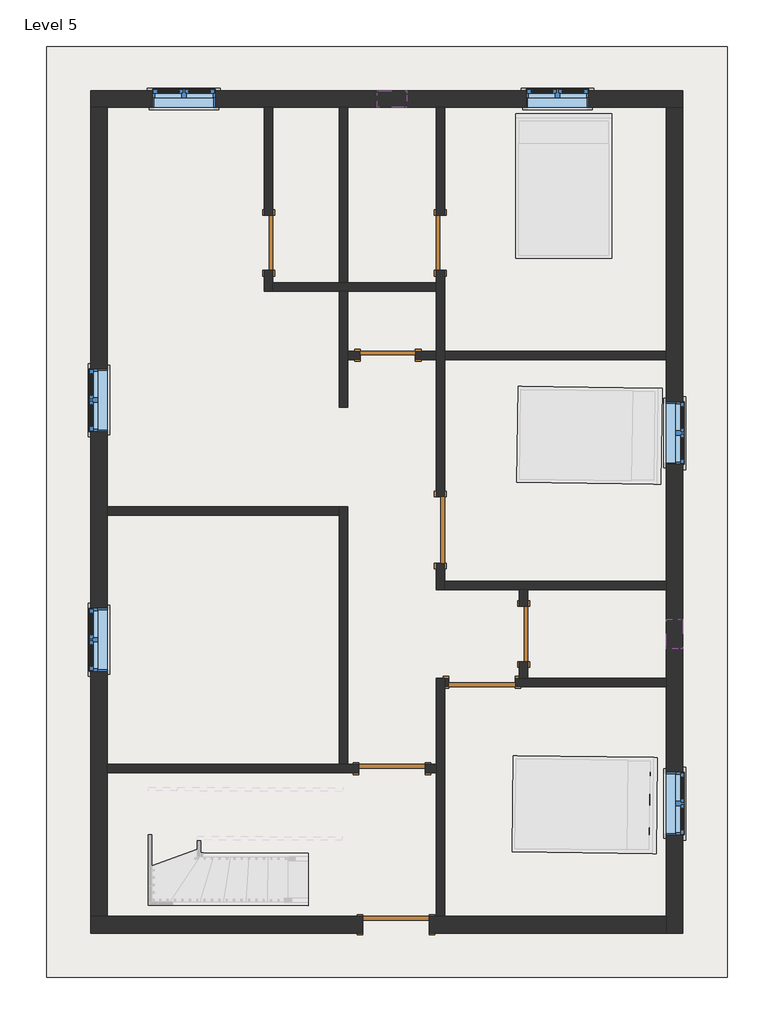
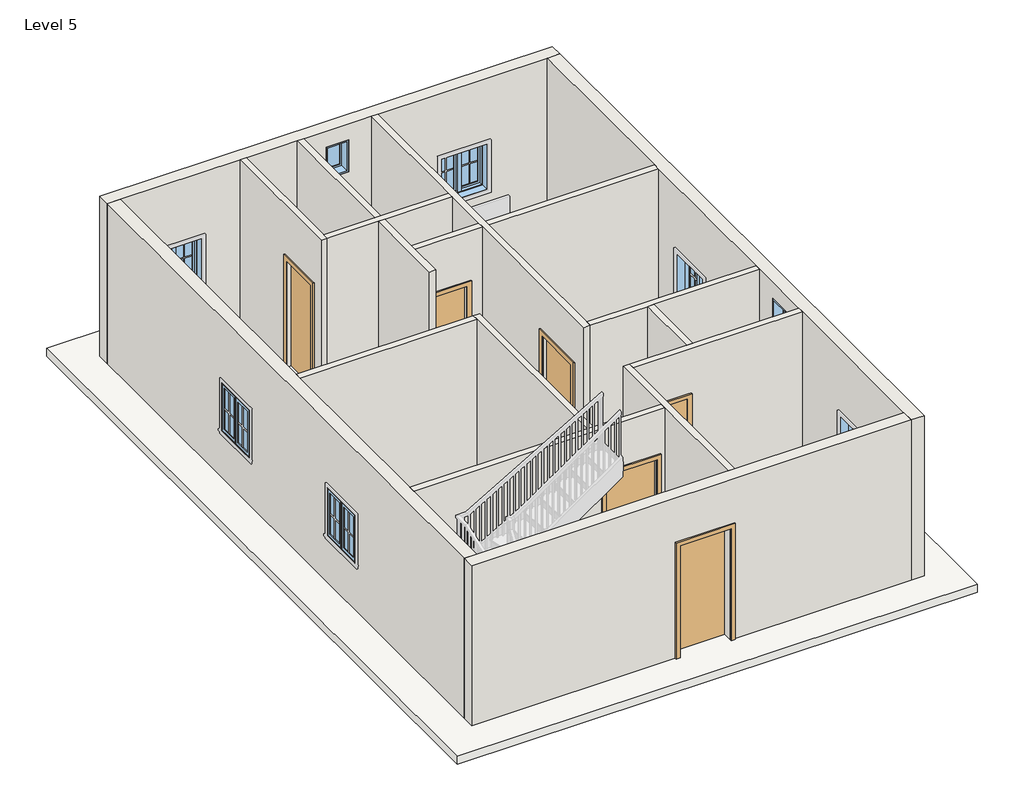
# One storey, part 1 of 3: 17 walls, 8 doors, 8 windows, 1 roof.
"""IFC4 building model written with IfcOpenShell, lengths in millimetres."""

from ifc_helpers import new_model, si_unit, frame, origin, place, context, project, spatial, polyline, outline, extrude, faceted_brep, transform, mapped, element, save
from components import door_d8f5dbb5, door_f2b275c1, door_e5f9f3c4, door_305aa2a5, door_0ca8825f, window_aa618e30, window_339605e1

model = new_model("IFC4")

# Units and contexts
model_context = context("Model", 3, world=origin())
ifc_project = project(units=[si_unit("LENGTHUNIT", "METRE", prefix="MILLI")], contexts=[model_context])

# Site, building, storey
site = spatial("IfcSite", under=ifc_project)
building = spatial("IfcBuilding", under=site)
storey = spatial("IfcBuildingStorey", under=building, Name="Level 5", Elevation=9601.2)

# Doors
placement = place(None, origin())
door_shape = door_d8f5dbb5(model_context)
element("IfcDoor", 1, ObjectType="Single-Flush : 30\" x 80\"", at=placement, inside=storey, context=model_context, shape_type="MappedRepresentation", body=[
    mapped(door_shape, transform((-2883.8867314, 4242.0321212, 9601.2), x_axis=(0.0, -1.0, 0.0), y_axis=(1.0, 0.0, 0.0), z_axis=(0.0, 0.0, 1.0))),
])
door_2_shape = door_f2b275c1(model_context)
element("IfcDoor", 2, ObjectType="Single-Flush : 30\" x 80\"", at=placement, inside=storey, context=model_context, shape_type="MappedRepresentation", body=[
    mapped(door_2_shape, transform((-521.6867314, 4242.0321212, 9601.2), x_axis=(0.0, -1.0, 0.0), y_axis=(1.0, 0.0, 0.0), z_axis=(0.0, 0.0, 1.0))),
])
element("IfcDoor", 3, ObjectType="Single-Flush : 30\" x 80\"", at=placement, inside=storey, context=model_context, shape_type="MappedRepresentation", body=[
    mapped(door_2_shape, transform((-1245.5867314, 2692.6321212, 9601.2), x_axis=(-1.0, 0.0, 0.0), y_axis=(0.0, -1.0, 0.0), z_axis=(0.0, 0.0, 1.0))),
])
element("IfcDoor", 4, ObjectType="Single-Flush : 30\" x 80\"", at=placement, inside=storey, context=model_context, shape_type="MappedRepresentation", body=[
    mapped(door_2_shape, transform((621.3132686, -1136.4178788, 9601.2), x_axis=(0.0, 1.0, 0.0), y_axis=(-1.0, 0.0, 0.0), z_axis=(0.0, 0.0, 1.0))),
])
door_3_shape = door_e5f9f3c4(model_context)
element("IfcDoor", 5, ObjectType="Single-Flush : 36\" x 84\"", at=placement, inside=storey, context=model_context, shape_type="MappedRepresentation", body=[
    mapped(door_3_shape, transform((-521.6867314, 292.3321212, 9601.2), x_axis=(0.0, -1.0, 0.0), y_axis=(1.0, 0.0, 0.0), z_axis=(0.0, 0.0, 1.0))),
])
element("IfcDoor", 6, ObjectType="Single-Flush : 36\" x 84\"", at=placement, inside=storey, context=model_context, shape_type="MappedRepresentation", body=[
    mapped(door_3_shape, transform((-1188.4367314, -2989.1542682, 9601.2), x_axis=(1.0, 0.0, 0.0), y_axis=(0.0, 1.0, 0.0), z_axis=(0.0, 0.0, 1.0))),
])
door_4_shape = door_305aa2a5(model_context)
element("IfcDoor", 7, ObjectType="Single-Flush : 36\" x 84\"", at=placement, inside=storey, context=model_context, shape_type="MappedRepresentation", body=[
    mapped(door_4_shape, transform((49.8132686, -1803.1678788, 9601.2), x_axis=(1.0, 0.0, 0.0), y_axis=(0.0, 1.0, 0.0), z_axis=(0.0, 0.0, 1.0))),
])
door_5_shape = door_0ca8825f(model_context)
element("IfcDoor", 8, ObjectType="Single-Flush : 36\" x 84\"", at=placement, inside=storey, context=model_context, shape_type="MappedRepresentation", body=[
    mapped(door_5_shape, transform((-1131.2867314, -5136.9178788, 9601.2), x_axis=(1.0, 0.0, 0.0), y_axis=(0.0, 1.0, 0.0), z_axis=(0.0, 0.0, 1.0))),
])

# Roof
element("IfcRoof", 9, ObjectType="Generic - 12\"", at=placement, inside=storey, context=model_context, shape_type="SweptSolid", body=[
    extrude(outline(polyline([(-5938.2367314, 6940.7821212), (3421.6632686, 6940.7821212), (3421.6632686, -5860.8178788), (-5938.2367314, -5860.8178788), (-5938.2367314, 6940.7821212)])), frame((0.0, 0.0, 9448.8), z_axis=(0.0, 0.0, 1.0), x_axis=(1.0, 0.0, 0.0)), (0.0, 0.0, 1.0), 152.4),
])

# Walls
element("IfcWall", 10, ObjectType="wall4.5\"", at=placement, inside=storey, context=model_context, shape_type="Brep", body=[
    faceted_brep([(-2941.0367314, 3861.0321212, 11633.2), (-2941.0367314, 3861.0321212, 9601.2), (-2941.0367314, 3575.2821212, 9601.2), (-2941.0367314, 3575.2821212, 12649.2), (-2941.0367314, 6102.5821212, 12649.2), (-2941.0367314, 6102.5821212, 9601.2), (-2941.0367314, 4623.0321212, 9601.2), (-2941.0367314, 4623.0321212, 11633.2), (-2826.7367314, 3575.2821212, 9601.2), (-2826.7367314, 3689.5821212, 9601.2), (-2826.7367314, 3861.0321212, 9601.2), (-2826.7367314, 3861.0321212, 11633.2), (-2826.7367314, 4623.0321212, 11633.2), (-2826.7367314, 4623.0321212, 9601.2), (-2826.7367314, 6102.5821212, 9601.2), (-2826.7367314, 6102.5821212, 12649.2), (-2826.7367314, 3689.5821212, 12649.2), (-2826.7367314, 3575.2821212, 12649.2)], [[[0, 1, 2, 3, 4, 5, 6, 7]], [[8, 9, 10, 11, 12, 13, 14, 15, 16, 17]], [[6, 5, 14, 13]], [[2, 1, 10, 9, 8]], [[5, 4, 15, 14]], [[3, 2, 8, 17]], [[11, 10, 1, 0]], [[12, 11, 0, 7]], [[13, 12, 7, 6]], [[4, 3, 17, 16, 15]]]),
])
element("IfcWall", 11, ObjectType="wall4.5\"", at=placement, inside=storey, context=model_context, shape_type="Brep", body=[
    faceted_brep([(-2826.7367314, 3575.2821212, 9601.2), (-1912.3367314, 3575.2821212, 9601.2), (-1798.0367314, 3575.2821212, 9601.2), (-578.8367314, 3575.2821212, 9601.2), (-578.8367314, 3575.2821212, 12649.2), (-1798.0367314, 3575.2821212, 12649.2), (-1912.3367314, 3575.2821212, 12649.2), (-2826.7367314, 3575.2821212, 12649.2), (-2826.7367314, 3689.5821212, 9601.2), (-2826.7367314, 3689.5821212, 12649.2), (-1912.3367314, 3689.5821212, 12649.2), (-1798.0367314, 3689.5821212, 12649.2), (-578.8367314, 3689.5821212, 12649.2), (-578.8367314, 3689.5821212, 9601.2), (-1798.0367314, 3689.5821212, 9601.2), (-1912.3367314, 3689.5821212, 9601.2)], [[[0, 1, 2, 3, 4, 5, 6, 7]], [[8, 9, 10, 11, 12, 13, 14, 15]], [[3, 2, 1, 0, 8, 15, 14, 13]], [[0, 7, 9, 8]], [[4, 3, 13, 12]], [[7, 6, 5, 4, 12, 11, 10, 9]]]),
])
element("IfcWall", 12, ObjectType="wall4.5\"", at=placement, inside=storey, context=model_context, shape_type="SweptSolid", body=[
    extrude(outline(polyline([(-1912.3367314, 3689.5821212), (-1912.3367314, 6102.5821212), (-1798.0367314, 6102.5821212), (-1798.0367314, 3689.5821212), (-1912.3367314, 3689.5821212)])), frame((0.0, 0.0, 9601.2), z_axis=(0.0, 0.0, 1.0), x_axis=(1.0, 0.0, 0.0)), (0.0, 0.0, 1.0), 3048.0),
])
element("IfcWall", 13, ObjectType="wall4.5\"", at=placement, inside=storey, context=model_context, shape_type="Brep", body=[
    faceted_brep([(-578.8367314, -164.8678788, 11734.8), (-578.8367314, -164.8678788, 9601.2), (-578.8367314, -526.8178788, 9601.2), (-578.8367314, -526.8178788, 12649.2), (-578.8367314, 2635.4821212, 12649.2), (-578.8367314, 2749.7821212, 12649.2), (-578.8367314, 3575.2821212, 12649.2), (-578.8367314, 3689.5821212, 12649.2), (-578.8367314, 6102.5821212, 12649.2), (-578.8367314, 6102.5821212, 9601.2), (-578.8367314, 4623.0321212, 9601.2), (-578.8367314, 4623.0321212, 11633.2), (-578.8367314, 3861.0321212, 11633.2), (-578.8367314, 3861.0321212, 9601.2), (-578.8367314, 3689.5821212, 9601.2), (-578.8367314, 3575.2821212, 9601.2), (-578.8367314, 2749.7821212, 9601.2), (-578.8367314, 2635.4821212, 9601.2), (-578.8367314, 749.5321212, 9601.2), (-578.8367314, 749.5321212, 11734.8), (-464.5367314, -526.8178788, 9601.2), (-464.5367314, -412.5178788, 9601.2), (-464.5367314, -164.8678788, 9601.2), (-464.5367314, -164.8678788, 11734.8), (-464.5367314, 749.5321212, 11734.8), (-464.5367314, 749.5321212, 9601.2), (-464.5367314, 2635.4821212, 9601.2), (-464.5367314, 2749.7821212, 9601.2), (-464.5367314, 3861.0321212, 9601.2), (-464.5367314, 3861.0321212, 11633.2), (-464.5367314, 4623.0321212, 11633.2), (-464.5367314, 4623.0321212, 9601.2), (-464.5367314, 6102.5821212, 9601.2), (-464.5367314, 6102.5821212, 12649.2), (-464.5367314, 2749.7821212, 12649.2), (-464.5367314, 2635.4821212, 12649.2), (-464.5367314, -412.5178788, 12649.2), (-464.5367314, -526.8178788, 12649.2)], [[[0, 1, 2, 3, 4, 5, 6, 7, 8, 9, 10, 11, 12, 13, 14, 15, 16, 17, 18, 19]], [[20, 21, 22, 23, 24, 25, 26, 27, 28, 29, 30, 31, 32, 33, 34, 35, 36, 37]], [[10, 9, 32, 31]], [[2, 1, 22, 21, 20]], [[18, 17, 16, 15, 14, 13, 28, 27, 26, 25]], [[9, 8, 33, 32]], [[3, 2, 20, 37]], [[29, 28, 13, 12]], [[30, 29, 12, 11]], [[31, 30, 11, 10]], [[23, 22, 1, 0]], [[24, 23, 0, 19]], [[25, 24, 19, 18]], [[8, 7, 6, 5, 4, 3, 37, 36, 35, 34, 33]]]),
])
element("IfcWall", 14, ObjectType="wall4.5\"", at=placement, inside=storey, context=model_context, shape_type="Brep", body=[
    faceted_brep([(-464.5367314, -526.8178788, 9601.2), (564.1632686, -526.8178788, 9601.2), (678.4632686, -526.8178788, 9601.2), (2583.4632686, -526.8178788, 9601.2), (2583.4632686, -526.8178788, 12649.2), (678.4632686, -526.8178788, 12649.2), (564.1632686, -526.8178788, 12649.2), (-464.5367314, -526.8178788, 12649.2), (-464.5367314, -412.5178788, 9601.2), (-464.5367314, -412.5178788, 12649.2), (2583.4632686, -412.5178788, 12649.2), (2583.4632686, -412.5178788, 9601.2)], [[[0, 1, 2, 3, 4, 5, 6, 7]], [[8, 9, 10, 11]], [[3, 2, 1, 0, 8, 11]], [[0, 7, 9, 8]], [[4, 3, 11, 10]], [[7, 6, 5, 4, 10, 9]]]),
])
element("IfcWall", 15, ObjectType="wall4.5\"", at=placement, inside=storey, context=model_context, shape_type="SweptSolid", body=[
    extrude(outline(polyline([(2583.4632686, 2749.7821212), (2583.4632686, 2635.4821212), (-464.5367314, 2635.4821212), (-464.5367314, 2749.7821212), (2583.4632686, 2749.7821212)])), frame((0.0, 0.0, 9601.2), z_axis=(0.0, 0.0, 1.0), x_axis=(1.0, 0.0, 0.0)), (0.0, 0.0, 1.0), 3048.0),
    extrude(outline(polyline([(12649.2, -1798.0367314), (9601.2, -1798.0367314), (9601.2, -1626.5867314), (11633.2, -1626.5867314), (11633.2, -864.5867314), (9601.2, -864.5867314), (9601.2, -578.8367314), (12649.2, -578.8367314), (12649.2, -1798.0367314)])), frame((0.0, 2635.4821212, 0.0), z_axis=(0.0, 1.0, 0.0), x_axis=(0.0, 0.0, 1.0)), (0.0, 0.0, 1.0), 114.3),
])
element("IfcWall", 16, ObjectType="wall4.5\"", at=placement, inside=storey, context=model_context, shape_type="Brep", body=[
    faceted_brep([(-1912.3367314, 3575.2821212, 9601.2), (-1912.3367314, 1982.8957318, 9601.2), (-1912.3367314, 1982.8957318, 12649.2), (-1912.3367314, 3575.2821212, 12649.2), (-1798.0367314, 3575.2821212, 9601.2), (-1798.0367314, 3575.2821212, 12649.2), (-1798.0367314, 2749.7821212, 12649.2), (-1798.0367314, 2635.4821212, 12649.2), (-1798.0367314, 1982.8957318, 12649.2), (-1798.0367314, 1982.8957318, 9601.2), (-1798.0367314, 2635.4821212, 9601.2), (-1798.0367314, 2749.7821212, 9601.2)], [[[0, 1, 2, 3]], [[4, 5, 6, 7, 8, 9, 10, 11]], [[1, 0, 4, 11, 10, 9]], [[2, 1, 9, 8]], [[0, 3, 5, 4]], [[3, 2, 8, 7, 6, 5]]]),
])
element("IfcWall", 17, ObjectType="wall4.5\"", at=placement, inside=storey, context=model_context, shape_type="Brep", body=[
    faceted_brep([(-1912.3367314, 611.2957318, 9601.2), (-1912.3367314, 496.9957318, 9601.2), (-1912.3367314, -2932.0042682, 9601.2), (-1912.3367314, -2932.0042682, 12649.2), (-1912.3367314, 496.9957318, 12649.2), (-1912.3367314, 611.2957318, 12649.2), (-1798.0367314, 611.2957318, 9601.2), (-1798.0367314, 611.2957318, 12649.2), (-1798.0367314, -2932.0042682, 12649.2), (-1798.0367314, -2932.0042682, 9601.2)], [[[0, 1, 2, 3, 4, 5]], [[6, 7, 8, 9]], [[2, 1, 0, 6, 9]], [[3, 2, 9, 8]], [[0, 5, 7, 6]], [[5, 4, 3, 8, 7]]]),
])
element("IfcWall", 18, ObjectType="wall4.5\"", at=placement, inside=storey, context=model_context, shape_type="Brep", body=[
    faceted_brep([(-731.2367314, -3046.3042682, 11734.8), (-731.2367314, -3046.3042682, 9601.2), (-578.8367314, -3046.3042682, 9601.2), (-578.8367314, -3046.3042682, 12649.2), (-5100.0367314, -3046.3042682, 12649.2), (-5100.0367314, -3046.3042682, 9601.2), (-1645.6367314, -3046.3042682, 9601.2), (-1645.6367314, -3046.3042682, 11734.8), (-578.8367314, -2932.0042682, 9601.2), (-731.2367314, -2932.0042682, 9601.2), (-731.2367314, -2932.0042682, 11734.8), (-1645.6367314, -2932.0042682, 11734.8), (-1645.6367314, -2932.0042682, 9601.2), (-1798.0367314, -2932.0042682, 9601.2), (-1912.3367314, -2932.0042682, 9601.2), (-5100.0367314, -2932.0042682, 9601.2), (-5100.0367314, -2932.0042682, 12649.2), (-1912.3367314, -2932.0042682, 12649.2), (-1798.0367314, -2932.0042682, 12649.2), (-578.8367314, -2932.0042682, 12649.2)], [[[0, 1, 2, 3, 4, 5, 6, 7]], [[8, 9, 10, 11, 12, 13, 14, 15, 16, 17, 18, 19]], [[6, 5, 15, 14, 13, 12]], [[2, 1, 9, 8]], [[5, 4, 16, 15]], [[3, 2, 8, 19]], [[10, 9, 1, 0]], [[11, 10, 0, 7]], [[12, 11, 7, 6]], [[4, 3, 19, 18, 17, 16]]]),
])
element("IfcWall", 19, ObjectType="wall4.5\"", at=placement, inside=storey, context=model_context, shape_type="Brep", body=[
    faceted_brep([(-464.5367314, -5022.6178788, 9601.2), (-464.5367314, -1860.3178788, 9601.2), (-464.5367314, -1746.0178788, 9601.2), (-464.5367314, -1746.0178788, 12649.2), (-464.5367314, -1860.3178788, 12649.2), (-464.5367314, -5022.6178788, 12649.2), (-578.8367314, -5022.6178788, 9601.2), (-578.8367314, -5022.6178788, 12649.2), (-578.8367314, -3046.3042682, 12649.2), (-578.8367314, -2932.0042682, 12649.2), (-578.8367314, -1746.0178788, 12649.2), (-578.8367314, -1746.0178788, 9601.2), (-578.8367314, -2932.0042682, 9601.2), (-578.8367314, -3046.3042682, 9601.2)], [[[0, 1, 2, 3, 4, 5]], [[6, 7, 8, 9, 10, 11, 12, 13]], [[2, 1, 0, 6, 13, 12, 11]], [[0, 5, 7, 6]], [[3, 2, 11, 10]], [[5, 4, 3, 10, 9, 8, 7]]]),
])
element("IfcWall", 20, ObjectType="wall4.5\"", at=placement, inside=storey, context=model_context, shape_type="Brep", body=[
    faceted_brep([(507.0132686, -1860.3178788, 11734.8), (507.0132686, -1860.3178788, 9601.2), (2583.4632686, -1860.3178788, 9601.2), (2583.4632686, -1860.3178788, 12649.2), (-464.5367314, -1860.3178788, 12649.2), (-464.5367314, -1860.3178788, 9601.2), (-407.3867314, -1860.3178788, 9601.2), (-407.3867314, -1860.3178788, 11734.8), (2583.4632686, -1746.0178788, 9601.2), (678.4632686, -1746.0178788, 9601.2), (564.1632686, -1746.0178788, 9601.2), (507.0132686, -1746.0178788, 9601.2), (507.0132686, -1746.0178788, 11734.8), (-407.3867314, -1746.0178788, 11734.8), (-407.3867314, -1746.0178788, 9601.2), (-464.5367314, -1746.0178788, 9601.2), (-464.5367314, -1746.0178788, 12649.2), (564.1632686, -1746.0178788, 12649.2), (678.4632686, -1746.0178788, 12649.2), (2583.4632686, -1746.0178788, 12649.2)], [[[0, 1, 2, 3, 4, 5, 6, 7]], [[8, 9, 10, 11, 12, 13, 14, 15, 16, 17, 18, 19]], [[6, 5, 15, 14]], [[2, 1, 11, 10, 9, 8]], [[5, 4, 16, 15]], [[3, 2, 8, 19]], [[12, 11, 1, 0]], [[13, 12, 0, 7]], [[14, 13, 7, 6]], [[4, 3, 19, 18, 17, 16]]]),
])
element("IfcWall", 21, ObjectType="wall4.5\"", at=placement, inside=storey, context=model_context, shape_type="SweptSolid", body=[
    extrude(outline(polyline([(-526.8178788, 9601.2), (-755.4178788, 9601.2), (-755.4178788, 11633.2), (-1517.4178788, 11633.2), (-1517.4178788, 9601.2), (-1746.0178788, 9601.2), (-1746.0178788, 12649.2), (-526.8178788, 12649.2), (-526.8178788, 9601.2)])), frame((564.1632686, 0.0, 0.0), z_axis=(1.0, 0.0, 0.0), x_axis=(0.0, 1.0, 0.0)), (0.0, 0.0, 1.0), 114.3),
])
element("IfcWall", 22, ObjectType="wall4.5\"", at=placement, inside=storey, context=model_context, shape_type="SweptSolid", body=[
    extrude(outline(polyline([(-5100.0367314, 611.2957318), (-1912.3367314, 611.2957318), (-1912.3367314, 496.9957318), (-5100.0367314, 496.9957318), (-5100.0367314, 611.2957318)])), frame((0.0, 0.0, 9601.2), z_axis=(0.0, 0.0, 1.0), x_axis=(1.0, 0.0, 0.0)), (0.0, 0.0, 1.0), 3048.0),
])
element("IfcWall", 23, ObjectType="wall9\"", at=placement, inside=storey, context=model_context, shape_type="Brep", body=[
    faceted_brep([(-5328.6367314, 6102.5821212, 9601.2), (-5100.0367314, 6102.5821212, 9601.2), (-2941.0367314, 6102.5821212, 9601.2), (-2826.7367314, 6102.5821212, 9601.2), (-1912.3367314, 6102.5821212, 9601.2), (-1798.0367314, 6102.5821212, 9601.2), (-578.8367314, 6102.5821212, 9601.2), (-464.5367314, 6102.5821212, 9601.2), (2583.4632686, 6102.5821212, 9601.2), (2812.0632686, 6102.5821212, 9601.2), (2812.0632686, 6102.5821212, 12649.2), (2583.4632686, 6102.5821212, 12649.2), (-464.5367314, 6102.5821212, 12649.2), (-578.8367314, 6102.5821212, 12649.2), (-1798.0367314, 6102.5821212, 12649.2), (-1912.3367314, 6102.5821212, 12649.2), (-2826.7367314, 6102.5821212, 12649.2), (-2941.0367314, 6102.5821212, 12649.2), (-5100.0367314, 6102.5821212, 12649.2), (-5328.6367314, 6102.5821212, 12649.2), (-985.2367314, 6102.5821212, 12344.4), (-985.2367314, 6102.5821212, 11734.8), (-1391.6367314, 6102.5821212, 11734.8), (-1391.6367314, 6102.5821212, 12344.4), (1519.8382686, 6102.5821212, 11430.0), (1519.8382686, 6102.5821212, 10515.6), (656.2382686, 6102.5821212, 10515.6), (656.2382686, 6102.5821212, 11430.0), (-3617.3117314, 6102.5821212, 11430.0), (-3617.3117314, 6102.5821212, 10515.6), (-4480.9117314, 6102.5821212, 10515.6), (-4480.9117314, 6102.5821212, 11430.0), (-5328.6367314, 6331.1821212, 9601.2), (-5328.6367314, 6331.1821212, 12649.2), (2812.0632686, 6331.1821212, 12649.2), (2812.0632686, 6331.1821212, 9601.2), (-985.2367314, 6331.1821212, 12344.4), (-1391.6367314, 6331.1821212, 12344.4), (-1391.6367314, 6331.1821212, 11734.8), (-985.2367314, 6331.1821212, 11734.8), (1519.8382686, 6331.1821212, 11430.0), (656.2382686, 6331.1821212, 11430.0), (656.2382686, 6331.1821212, 10515.6), (1519.8382686, 6331.1821212, 10515.6), (-3617.3117314, 6331.1821212, 11430.0), (-4480.9117314, 6331.1821212, 11430.0), (-4480.9117314, 6331.1821212, 10515.6), (-3617.3117314, 6331.1821212, 10515.6)], [[[0, 1, 2, 3, 4, 5, 6, 7, 8, 9, 10, 11, 12, 13, 14, 15, 16, 17, 18, 19], [20, 21, 22, 23], [24, 25, 26, 27], [28, 29, 30, 31]], [[32, 33, 34, 35], [36, 37, 38, 39], [40, 41, 42, 43], [44, 45, 46, 47]], [[9, 8, 7, 6, 5, 4, 3, 2, 1, 0, 32, 35]], [[10, 9, 35, 34]], [[0, 19, 33, 32]], [[21, 20, 36, 39]], [[22, 21, 39, 38]], [[23, 22, 38, 37]], [[20, 23, 37, 36]], [[25, 24, 40, 43]], [[26, 25, 43, 42]], [[27, 26, 42, 41]], [[24, 27, 41, 40]], [[29, 28, 44, 47]], [[30, 29, 47, 46]], [[31, 30, 46, 45]], [[28, 31, 45, 44]], [[19, 18, 17, 16, 15, 14, 13, 12, 11, 10, 34, 33]]]),
])
element("IfcWall", 24, ObjectType="wall9\"", at=placement, inside=storey, context=model_context, shape_type="Brep", body=[
    faceted_brep([(2583.4632686, 6102.5821212, 9601.2), (2583.4632686, 2749.7821212, 9601.2), (2583.4632686, 2635.4821212, 9601.2), (2583.4632686, -412.5178788, 9601.2), (2583.4632686, -526.8178788, 9601.2), (2583.4632686, -1746.0178788, 9601.2), (2583.4632686, -1860.3178788, 9601.2), (2583.4632686, -5022.6178788, 9601.2), (2583.4632686, -5251.2178788, 9601.2), (2583.4632686, -5251.2178788, 12649.2), (2583.4632686, -5022.6178788, 12649.2), (2583.4632686, -1860.3178788, 12649.2), (2583.4632686, -1746.0178788, 12649.2), (2583.4632686, -526.8178788, 12649.2), (2583.4632686, -412.5178788, 12649.2), (2583.4632686, 2635.4821212, 12649.2), (2583.4632686, 2749.7821212, 12649.2), (2583.4632686, 6102.5821212, 12649.2), (2583.4632686, -1339.6178788, 12344.4), (2583.4632686, -1339.6178788, 11734.8), (2583.4632686, -933.2178788, 11734.8), (2583.4632686, -933.2178788, 12344.4), (2583.4632686, 1194.0321212, 11430.0), (2583.4632686, 1194.0321212, 10515.6), (2583.4632686, 2057.6321212, 10515.6), (2583.4632686, 2057.6321212, 11430.0), (2583.4632686, -3901.8428788, 11430.0), (2583.4632686, -3901.8428788, 10515.6), (2583.4632686, -3038.2428788, 10515.6), (2583.4632686, -3038.2428788, 11430.0), (2812.0632686, 6102.5821212, 9601.2), (2812.0632686, 6102.5821212, 12649.2), (2812.0632686, -5251.2178788, 12649.2), (2812.0632686, -5251.2178788, 9601.2), (2812.0632686, -1339.6178788, 12344.4), (2812.0632686, -933.2178788, 12344.4), (2812.0632686, -933.2178788, 11734.8), (2812.0632686, -1339.6178788, 11734.8), (2812.0632686, 1194.0321212, 11430.0), (2812.0632686, 2057.6321212, 11430.0), (2812.0632686, 2057.6321212, 10515.6), (2812.0632686, 1194.0321212, 10515.6), (2812.0632686, -3901.8428788, 11430.0), (2812.0632686, -3038.2428788, 11430.0), (2812.0632686, -3038.2428788, 10515.6), (2812.0632686, -3901.8428788, 10515.6)], [[[0, 1, 2, 3, 4, 5, 6, 7, 8, 9, 10, 11, 12, 13, 14, 15, 16, 17], [18, 19, 20, 21], [22, 23, 24, 25], [26, 27, 28, 29]], [[30, 31, 32, 33], [34, 35, 36, 37], [38, 39, 40, 41], [42, 43, 44, 45]], [[8, 7, 6, 5, 4, 3, 2, 1, 0, 30, 33]], [[0, 17, 31, 30]], [[9, 8, 33, 32]], [[19, 18, 34, 37]], [[20, 19, 37, 36]], [[21, 20, 36, 35]], [[18, 21, 35, 34]], [[23, 22, 38, 41]], [[24, 23, 41, 40]], [[25, 24, 40, 39]], [[22, 25, 39, 38]], [[27, 26, 42, 45]], [[28, 27, 45, 44]], [[29, 28, 44, 43]], [[26, 29, 43, 42]], [[17, 16, 15, 14, 13, 12, 11, 10, 9, 32, 31]]]),
])
element("IfcWall", 25, ObjectType="wall9\"", at=placement, inside=storey, context=model_context, shape_type="Brep", body=[
    faceted_brep([(2583.4632686, -5022.6178788, 9601.2), (-464.5367314, -5022.6178788, 9601.2), (-578.8367314, -5022.6178788, 9601.2), (-674.0867314, -5022.6178788, 9601.2), (-674.0867314, -5022.6178788, 11734.8), (-1588.4867314, -5022.6178788, 11734.8), (-1588.4867314, -5022.6178788, 9601.2), (-5100.0367314, -5022.6178788, 9601.2), (-5328.6367314, -5022.6178788, 9601.2), (-5328.6367314, -5022.6178788, 12649.2), (-5100.0367314, -5022.6178788, 12649.2), (-578.8367314, -5022.6178788, 12649.2), (-464.5367314, -5022.6178788, 12649.2), (2583.4632686, -5022.6178788, 12649.2), (-674.0867314, -5251.2178788, 11734.8), (-674.0867314, -5251.2178788, 9601.2), (2583.4632686, -5251.2178788, 9601.2), (2583.4632686, -5251.2178788, 12649.2), (-5328.6367314, -5251.2178788, 12649.2), (-5328.6367314, -5251.2178788, 9601.2), (-1588.4867314, -5251.2178788, 9601.2), (-1588.4867314, -5251.2178788, 11734.8)], [[[0, 1, 2, 3, 4, 5, 6, 7, 8, 9, 10, 11, 12, 13]], [[14, 15, 16, 17, 18, 19, 20, 21]], [[20, 19, 8, 7, 6]], [[16, 15, 3, 2, 1, 0]], [[0, 13, 17, 16]], [[9, 8, 19, 18]], [[4, 3, 15, 14]], [[5, 4, 14, 21]], [[6, 5, 21, 20]], [[13, 12, 11, 10, 9, 18, 17]]]),
])
element("IfcWall", 26, ObjectType="wall9\"", at=placement, inside=storey, context=model_context, shape_type="Brep", body=[
    faceted_brep([(-5328.6367314, 6102.5821212, 9601.2), (-5328.6367314, -5022.6178788, 9601.2), (-5328.6367314, -5022.6178788, 12649.2), (-5328.6367314, 6102.5821212, 12649.2), (-5328.6367314, 2509.9457318, 11430.0), (-5328.6367314, 1646.3457318, 11430.0), (-5328.6367314, 1646.3457318, 10515.6), (-5328.6367314, 2509.9457318, 10515.6), (-5328.6367314, -785.7042682, 11430.0), (-5328.6367314, -1649.3042682, 11430.0), (-5328.6367314, -1649.3042682, 10515.6), (-5328.6367314, -785.7042682, 10515.6), (-5100.0367314, 6102.5821212, 9601.2), (-5100.0367314, 6102.5821212, 12649.2), (-5100.0367314, 611.2957318, 12649.2), (-5100.0367314, 496.9957318, 12649.2), (-5100.0367314, -2932.0042682, 12649.2), (-5100.0367314, -3046.3042682, 12649.2), (-5100.0367314, -5022.6178788, 12649.2), (-5100.0367314, -5022.6178788, 9601.2), (-5100.0367314, -3046.3042682, 9601.2), (-5100.0367314, -2932.0042682, 9601.2), (-5100.0367314, 496.9957318, 9601.2), (-5100.0367314, 611.2957318, 9601.2), (-5100.0367314, 2509.9457318, 11430.0), (-5100.0367314, 2509.9457318, 10515.6), (-5100.0367314, 1646.3457318, 10515.6), (-5100.0367314, 1646.3457318, 11430.0), (-5100.0367314, -785.7042682, 11430.0), (-5100.0367314, -785.7042682, 10515.6), (-5100.0367314, -1649.3042682, 10515.6), (-5100.0367314, -1649.3042682, 11430.0)], [[[0, 1, 2, 3], [4, 5, 6, 7], [8, 9, 10, 11]], [[12, 13, 14, 15, 16, 17, 18, 19, 20, 21, 22, 23], [24, 25, 26, 27], [28, 29, 30, 31]], [[1, 0, 12, 23, 22, 21, 20, 19]], [[0, 3, 13, 12]], [[2, 1, 19, 18]], [[25, 24, 4, 7]], [[26, 25, 7, 6]], [[27, 26, 6, 5]], [[24, 27, 5, 4]], [[29, 28, 8, 11]], [[30, 29, 11, 10]], [[31, 30, 10, 9]], [[28, 31, 9, 8]], [[3, 2, 18, 17, 16, 15, 14, 13]]]),
])

# Windows
window_shape = window_aa618e30(model_context)
element("IfcWindow", 27, ObjectType="Fixed : 16\" x 24\"", at=placement, inside=storey, context=model_context, shape_type="MappedRepresentation", body=[
    mapped(window_shape, transform((-1150.3367314, 6216.8821212, 10820.4), x_axis=(1.0, 0.0, 0.0), y_axis=(0.0, 1.0, 0.0), z_axis=(0.0, 0.0, 1.0))),
])
element("IfcWindow", 28, ObjectType="Fixed : 16\" x 24\"", at=placement, inside=storey, context=model_context, shape_type="MappedRepresentation", body=[
    mapped(window_shape, transform((2697.7632686, -1174.5178788, 10820.4), x_axis=(0.0, -1.0, 0.0), y_axis=(1.0, 0.0, 0.0), z_axis=(0.0, 0.0, 1.0))),
])
window_2_shape = window_339605e1(model_context)
element("IfcWindow", 29, ObjectType="Window-Casement-Double : 34\" x 36\"", at=placement, inside=storey, context=model_context, shape_type="MappedRepresentation", body=[
    mapped(window_2_shape, transform((1088.0382686, 6216.8821212, 9601.2), x_axis=(1.0, 0.0, 0.0), y_axis=(0.0, 1.0, 0.0), z_axis=(0.0, 0.0, 1.0))),
])
element("IfcWindow", 30, ObjectType="Window-Casement-Double : 34\" x 36\"", at=placement, inside=storey, context=model_context, shape_type="MappedRepresentation", body=[
    mapped(window_2_shape, transform((2697.7632686, 1625.8321212, 9601.2), x_axis=(0.0, -1.0, 0.0), y_axis=(1.0, 0.0, 0.0), z_axis=(0.0, 0.0, 1.0))),
])
element("IfcWindow", 31, ObjectType="Window-Casement-Double : 34\" x 36\"", at=placement, inside=storey, context=model_context, shape_type="MappedRepresentation", body=[
    mapped(window_2_shape, transform((2697.7632686, -3470.0428788, 9601.2), x_axis=(0.0, -1.0, 0.0), y_axis=(1.0, 0.0, 0.0), z_axis=(0.0, 0.0, 1.0))),
])
element("IfcWindow", 32, ObjectType="Window-Casement-Double : 34\" x 36\"", at=placement, inside=storey, context=model_context, shape_type="MappedRepresentation", body=[
    mapped(window_2_shape, transform((-4049.1117314, 6216.8821212, 9601.2), x_axis=(1.0, 0.0, 0.0), y_axis=(0.0, 1.0, 0.0), z_axis=(0.0, 0.0, 1.0))),
])
element("IfcWindow", 33, ObjectType="Window-Casement-Double : 34\" x 36\"", at=placement, inside=storey, context=model_context, shape_type="MappedRepresentation", body=[
    mapped(window_2_shape, transform((-5214.3367314, 2078.1457318, 9601.2), x_axis=(0.0, 1.0, 0.0), y_axis=(-1.0, 0.0, 0.0), z_axis=(0.0, 0.0, 1.0))),
])
element("IfcWindow", 34, ObjectType="Window-Casement-Double : 34\" x 36\"", at=placement, inside=storey, context=model_context, shape_type="MappedRepresentation", body=[
    mapped(window_2_shape, transform((-5214.3367314, -1217.5042682, 9601.2), x_axis=(0.0, 1.0, 0.0), y_axis=(-1.0, 0.0, 0.0), z_axis=(0.0, 0.0, 1.0))),
])

save(model, "model.ifc")

# Revit data of these elements
# Type "Single-Flush : 30\" x 80\""
#   Type Mark = "5"
#   Construction Type Id = "MDOOR"
#   Assembly Code = "C1020"
#   Analytic Construction = "Metal"
#   Thickness = 0' - 2"
#   Heat Transfer Coefficient (U) = 0.651978 BTU/(h·ft²·°F)
#   Height = 6' - 8"
#   Trim Projection Ext = 0' - 1"
#   Trim Projection Int = 0' - 1"
#   Trim Width = 0' - 3"
#   Width = 2' - 6"
#   Define Thermal Properties by = 1
#   Define Thermal Properties by = 1
#   Door Material = Door - Panel
#   Frame Material = Door - Frame
#   Visual Light Transmittance = 0
#   Solar Heat Gain Coefficient = 0
#   Function = (empty or 0)
#   Wall Closure = (empty or 0)
# Type "Single-Flush : 36\" x 84\""
#   Type Mark = "1"
#   Construction Type Id = "MDOOR"
#   Assembly Code = "C1020"
#   Analytic Construction = "Metal"
#   Thickness = 0' - 2"
#   Heat Transfer Coefficient (U) = 0.651978 BTU/(h·ft²·°F)
#   Height = 7' - 0"
#   Trim Projection Ext = 0' - 1"
#   Trim Projection Int = 0' - 1"
#   Trim Width = 0' - 3"
#   Width = 3' - 0"
#   Define Thermal Properties by = 1
#   Define Thermal Properties by = 1
#   Door Material = Door - Panel
#   Frame Material = Door - Frame
#   Visual Light Transmittance = 0
#   Solar Heat Gain Coefficient = 0
#   Function = (empty or 0)
#   Wall Closure = (empty or 0)
# Type "Generic - 12\""
#   Assembly Code = "B1020"
#   Layers, outside or top first: 0' - 6" no material (function 1)
# Type "wall4.5\""
#   Assembly Code = "B2010"
#   Layers, outside or top first: 0' - 4 1/2" no material (function 1)
# Type "wall9\""
#   Assembly Code = "B2010"
#   Layers, outside or top first: 0' - 9" no material (function 1)
# Type "Fixed : 16\" x 24\""
#   Type Mark = "4"
#   Construction Type Id = "GSP4R"
#   Assembly Code = "B2020100"
#   Analytic Construction = "1/8 in Pilkington single glazing"
#   Visual Light Transmittance = 0.9
#   Solar Heat Gain Coefficient = 0.78
#   Heat Transfer Coefficient (U) = 0.6496 BTU/(h·ft²·°F)
#   Height = 2' - 0"
#   Default Sill Height = 3' - 0"
#   Width = 1' - 4"
#   Window Inset = 0' - 0 3/4"
#   Define Thermal Properties by = 1
#   Define Thermal Properties by = 1
#   Glass Pane Material = Glass
#   Sash Material = Sash
#   Wall Closure = (empty or 0)
# Type "Window-Casement-Double : 34\" x 36\""
#   Type Mark = "14"
#   Fire Rating = "0.5h"
#   Assembly Code = "B2020100"
#   Analytic Construction = "Double glazing - domestic"
#   Frame Extension [instance default] = 0' - 0 1/4"
#   Window Inset [instance default] = 0' - 0"
#   Wall Thickness [instance default] = 0' - 6"
#   Interior Wall Closure [instance default] = 0' - 2 1/4"
#   Half Width = 1' - 5"
#   Visual Light Transmittance = 0.81
#   Thermal Resistance (R) = 1.8146 (h·ft²·°F)/BTU
#   Solar Heat Gain Coefficient = 0.76
#   Rough Width = 2' - 10 1/2"
#   Rough Height = 3' - 0 1/2"
#   Height = 3' - 0"
#   Heat Transfer Coefficient (U) = 0.5511 BTU/(h·ft²·°F)
#   Exterior Wall Closure [instance default] = 0' - 1 1/4"
#   Extension Jamb [instance default] = 0' - 2 1/4"
#   Default Sill Height = 3' - 0"
#   Width = 2' - 10"
#   Define Thermal Properties by = 0
#   Muntin Visibility = yes
#   Interior Trim Visibility [instance default] = yes
#   Exterior Trim Visibility [instance default] = yes
#   Extension Jamb Visibility [instance default] = yes
#   Interior Trim Material = Wood - Stained
#   Muntin Pattern = Muntin Pattern_2x2 : Muntin Pattern_2x2
#   Interior Trim = Trim-Window-Interior-Flat : Picture Frame
#   Interior Frame Material = Wood - Stained
#   Glass Panel Material = Glass
#   Exterior Trim Material = Clad - White
#   Exterior Trim = Trim-Window-Exterior-Flat : with Sill
#   Exterior Frame Material = Clad - White
#   Wall Closure = (empty or 0)
# Elements 1, 2, 3, 4 (IfcDoor, "Single-Flush : 30\" x 80\"")
#   Phase Created = New Construction
#   Materials on its faces: "Door - Frame", "Door - Panel"
# Elements 5, 6, 7, 8 (IfcDoor, "Single-Flush : 36\" x 84\"")
#   Phase Created = New Construction
#   Materials on its faces: "Door - Frame", "Door - Panel"
# Element 9 (IfcRoof, "Generic - 12\"")
#   built-in parameter 1001705 = 31.5 (stored number, unit not read)
#   built-in parameter 1001701 = -0.5 (stored number, unit not read)
#   built-in parameter 1001710 = 33615
#   Phase Created = New Construction
#   Materials on its faces: "Default Roof"
# Elements 10, 11, 12, 13, 14, 15, 16, 17, 18, 19, 20, 21, 22 (IfcWall, "wall4.5\"")
#   Top Offset = 0' - 0"
#   Base Offset = 0' - 0"
#   Unconnected Height = 10' - 0"
#   wall height = 10' - 0"
#   Phase Created = New Construction
#   Base Constraint = Level 5
#   Materials on its faces: "Default Wall"
# Elements 23, 24, 25, 26 (IfcWall, "wall9\"")
#   Top Offset = 0' - 0"
#   Base Offset = 0' - 0"
#   Unconnected Height = 10' - 0"
#   wall height = 10' - 0"
#   Phase Created = New Construction
#   Base Constraint = Level 5
#   Materials on its faces: "Default Wall", "Wood Planks"
# Element 27 (IfcWindow, "Fixed : 16\" x 24\"")
#   Mark = "25"
#   Phase Created = New Construction
#   Materials on its faces: "Sash", "Glass"
# Element 28 (IfcWindow, "Fixed : 16\" x 24\"")
#   Mark = "26"
#   Phase Created = New Construction
#   Materials on its faces: "Sash", "Glass"
# Element 29 (IfcWindow, "Window-Casement-Double : 34\" x 36\"")
#   Mark = "27"
#   Window Inset = 0' - 0"
#   Interior Wall Closure = 0' - 2 1/4"
#   Frame Extension = 0' - 0 1/4"
#   Exterior Wall Closure = 0' - 1 1/4"
#   Interior Trim Visibility = yes
#   Exterior Trim Visibility = yes
#   Phase Created = New Construction
#   Materials on its faces: "Wood - Stained", "Glass", "Clad - White"
# Element 30 (IfcWindow, "Window-Casement-Double : 34\" x 36\"")
#   Mark = "28"
#   Window Inset = 0' - 0"
#   Interior Wall Closure = 0' - 2 1/4"
#   Frame Extension = 0' - 0 1/4"
#   Exterior Wall Closure = 0' - 1 1/4"
#   Interior Trim Visibility = yes
#   Exterior Trim Visibility = yes
#   Phase Created = New Construction
#   Materials on its faces: "Wood - Stained", "Glass", "Clad - White"
# Element 31 (IfcWindow, "Window-Casement-Double : 34\" x 36\"")
#   Mark = "29"
#   Window Inset = 0' - 0"
#   Interior Wall Closure = 0' - 2 1/4"
#   Frame Extension = 0' - 0 1/4"
#   Exterior Wall Closure = 0' - 1 1/4"
#   Interior Trim Visibility = yes
#   Exterior Trim Visibility = yes
#   Phase Created = New Construction
#   Materials on its faces: "Wood - Stained", "Glass", "Clad - White"
# Element 32 (IfcWindow, "Window-Casement-Double : 34\" x 36\"")
#   Mark = "30"
#   Window Inset = 0' - 0"
#   Interior Wall Closure = 0' - 2 1/4"
#   Frame Extension = 0' - 0 1/4"
#   Exterior Wall Closure = 0' - 1 1/4"
#   Interior Trim Visibility = yes
#   Exterior Trim Visibility = yes
#   Phase Created = New Construction
#   Materials on its faces: "Wood - Stained", "Glass", "Clad - White"
# Element 33 (IfcWindow, "Window-Casement-Double : 34\" x 36\"")
#   Mark = "31"
#   Window Inset = 0' - 0"
#   Interior Wall Closure = 0' - 2 1/4"
#   Frame Extension = 0' - 0 1/4"
#   Exterior Wall Closure = 0' - 1 1/4"
#   Interior Trim Visibility = yes
#   Exterior Trim Visibility = yes
#   Phase Created = New Construction
#   Materials on its faces: "Wood - Stained", "Glass", "Clad - White"
# Element 34 (IfcWindow, "Window-Casement-Double : 34\" x 36\"")
#   Mark = "32"
#   Window Inset = 0' - 0"
#   Interior Wall Closure = 0' - 2 1/4"
#   Frame Extension = 0' - 0 1/4"
#   Exterior Wall Closure = 0' - 1 1/4"
#   Interior Trim Visibility = yes
#   Exterior Trim Visibility = yes
#   Phase Created = New Construction
#   Materials on its faces: "Wood - Stained", "Glass", "Clad - White"
# Materials
#   "Door - Panel": class "Wood", colour RGB 210 159 95, transparency 0, Cost = 0
#   "Door - Frame": colour RGB 118 70 51, transparency 0, Cost = 0
#   "Glass": class "Glass", colour RGB 0 128 192, transparency 0.75, Description = "Soda Lime Glass", Cost = 0
#   "Sash": class "Wood", colour RGB 224 178 126, transparency 0, Cost = 0
#   "Wood - Stained": class "Wood", colour RGB 224 178 126, transparency 0, Cost = 0
#   "Clad - White": class "Wood", colour RGB 242 242 238, transparency 0, Cost = 0
#   "Default Roof": colour RGB 88 101 114, transparency 0, Cost = 0
#   "Default Wall": colour RGB 128 128 128, transparency 0, Cost = 0
#   "Wood Planks": class "Wood", colour RGB 193 160 115, transparency 0, Description = "Physical material.", Cost = 0
